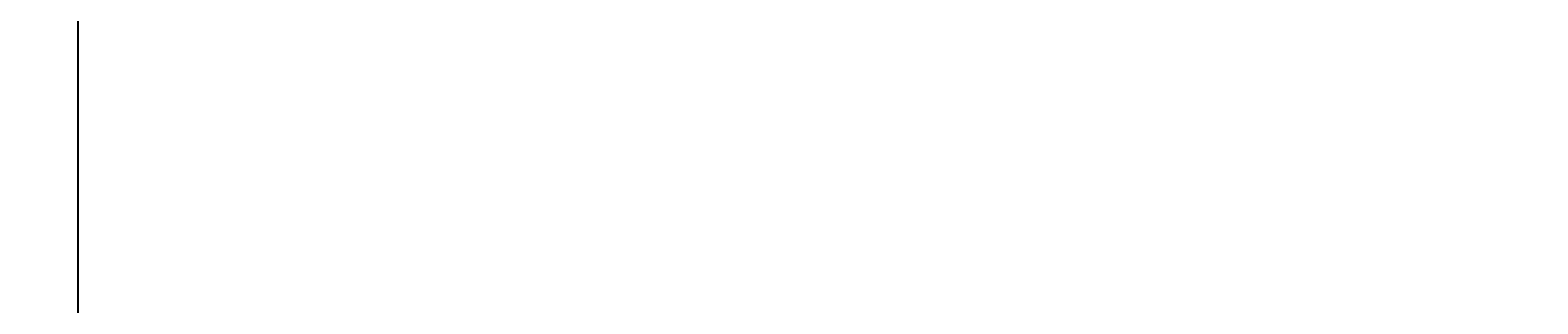
# Model space of a CAD drawing. Units: inches. Extents: x 35362 to 73946, y 43607 to 67532.
# Tile 104 of 134: x 50119 to 50761, y 49386 to 49502. Entities that reach past the tile are written whole.
import ezdxf

# ---------------------------------------------------------------- set-up
doc = ezdxf.new("R2010")
doc.units = ezdxf.units.IN
doc.header["$MEASUREMENT"] = 0
doc.layers.add('A-ANNO-DIMS', color=2, linetype='Continuous', lineweight=18)
doc.styles.get("Standard").update_dxf_attribs({"font": 'arial.ttf'})
doc.dimstyles.get("Standard").update_dxf_attribs({"dimtxt": 0.18, "dimasz": 0.18, "dimexe": 0.18, "dimexo": 0.0625, "dimgap": 0.09, "dimtad": 0, "dimtih": 1, "dimtoh": 1, "dimdec": 4, "dimzin": 0, "dimdsep": 46, "dimtxsty": 'Standard', "dimcen": 0.09, "dimadec": 0, "dimazin": 0, "dimtfac": 1, "dimtdec": 4, "dimtofl": 0, "dimtmove": 0, "dimatfit": 3, "dimfxl": 1, "dimtolj": 1, "dimtzin": 0, "dimarcsym": 0})

# ---------------------------------------------------------------- blocks, each defined once
blk = doc.blocks.new('*D11')
at = {"layer": 'A-ANNO-DIMS', "color": 0, "lineweight": -2, "transparency": 16777216}
for p, q in [((47978.66, 56028.77), (47978.66, 43606.68)), ((53109.76, 56028.77), (53109.76, 43606.68)), ((47978.84, 43606.86), (50543.87, 43606.86)), ((53109.58, 43606.86), (50544.55, 43606.86))]:
    blk.add_line(p, q, dxfattribs=at)
at = {"layer": 'A-ANNO-DIMS', "color": 0, "transparency": 16777216}
for points in [[(47978.84, 43606.89), (47978.84, 43606.83), (47978.66, 43606.86)], [(53109.58, 43606.89), (53109.58, 43606.83), (53109.76, 43606.86)]]:
    blk.add_solid(points, dxfattribs=at)
at = {"layer": 'Defpoints', "color": 0, "transparency": 16777216}
for p in [(47978.66, 56028.84), (53109.76, 56028.84), (53109.76, 43606.86)]:
    blk.add_point(p, dxfattribs=at)
at = {"layer": 'A-ANNO-DIMS', "color": 0, "transparency": 16777216, "insert": (50544.21, 43606.86), "char_height": 0.18, "attachment_point": 5}
blk.add_mtext('\\A1;5131', dxfattribs=at)
blk = doc.blocks.new('*D13')
at = {"layer": 'A-ANNO-DIMS', "color": 0, "lineweight": -2, "transparency": 16777216}
for p, q in [((48373.49, 51694.02), (48373.49, 43606.68)), ((51029.04, 51694.02), (51029.04, 43606.68)), ((48373.67, 43606.86), (49700.8, 43606.86)), ((51028.86, 43606.86), (49701.73, 43606.86))]:
    blk.add_line(p, q, dxfattribs=at)
at = {"layer": 'A-ANNO-DIMS', "color": 0, "transparency": 16777216}
for points in [[(48373.67, 43606.89), (48373.67, 43606.83), (48373.49, 43606.86)], [(51028.86, 43606.89), (51028.86, 43606.83), (51029.04, 43606.86)]]:
    blk.add_solid(points, dxfattribs=at)
at = {"layer": 'Defpoints', "color": 0, "transparency": 16777216}
for p in [(48373.49, 51694.09), (51029.04, 51694.09), (51029.04, 43606.86)]:
    blk.add_point(p, dxfattribs=at)
at = {"layer": 'A-ANNO-DIMS', "color": 0, "transparency": 16777216, "insert": (49701.27, 43606.86), "char_height": 0.18, "attachment_point": 5}
blk.add_mtext('\\A1;2655.6', dxfattribs=at)
blk = doc.blocks.new('*D17')
at = {"layer": 'A-ANNO-DIMS', "color": 0, "lineweight": -2, "transparency": 16777216}
for p, q in [((49923.31, 61293.22), (49923.31, 43606.68)), ((51913.93, 61293.22), (51913.93, 43606.68)), ((49923.49, 43606.86), (50918.16, 43606.86)), ((51913.75, 43606.86), (50919.07, 43606.86))]:
    blk.add_line(p, q, dxfattribs=at)
at = {"layer": 'A-ANNO-DIMS', "color": 0, "transparency": 16777216}
for points in [[(49923.49, 43606.89), (49923.49, 43606.83), (49923.31, 43606.86)], [(51913.75, 43606.89), (51913.75, 43606.83), (51913.93, 43606.86)]]:
    blk.add_solid(points, dxfattribs=at)
at = {"layer": 'Defpoints', "color": 0, "transparency": 16777216}
for p in [(49923.31, 61293.29), (51913.93, 61293.29), (51913.93, 43606.86)]:
    blk.add_point(p, dxfattribs=at)
at = {"layer": 'A-ANNO-DIMS', "color": 0, "transparency": 16777216, "insert": (50918.62, 43606.86), "char_height": 0.18, "attachment_point": 5}
blk.add_mtext('\\A1;1990.6', dxfattribs=at)
blk = doc.blocks.new('*D40')
at = {"layer": 'A-ANNO-DIMS', "color": 0, "lineweight": -2, "transparency": 16777216}
for p, q in [((56873.54, 53351.53), (35361.77, 53351.53)), ((35361.95, 53351.35), (35361.95, 51333.28)), ((35361.95, 49314.85), (35361.95, 51332.92)), ((51806.45, 49314.67), (35361.77, 49314.67))]:
    blk.add_line(p, q, dxfattribs=at)
at = {"layer": 'A-ANNO-DIMS', "color": 0, "transparency": 16777216}
for points in [[(35361.92, 53351.35), (35361.98, 53351.35), (35361.95, 53351.53)], [(35361.92, 49314.85), (35361.98, 49314.85), (35361.95, 49314.67)]]:
    blk.add_solid(points, dxfattribs=at)
at = {"layer": 'Defpoints', "color": 0, "transparency": 16777216}
for p in [(35361.95, 53351.53), (56873.6, 53351.53), (51806.52, 49314.67)]:
    blk.add_point(p, dxfattribs=at)
at = {"layer": 'A-ANNO-DIMS', "color": 0, "transparency": 16777216, "insert": (35361.95, 51333.1), "char_height": 0.18, "attachment_point": 5}
blk.add_mtext('\\A1;4036.9', dxfattribs=at)
blk = doc.blocks.new('*D67')
at = {"layer": 'A-ANNO-DIMS', "color": 0, "lineweight": -2, "transparency": 16777216}
for p, q in [((56873.54, 53351.53), (35361.77, 53351.53)), ((35361.95, 53351.35), (35361.95, 49400.89)), ((35361.95, 45450.07), (35361.95, 49400.53)), ((53793.58, 45449.89), (35361.77, 45449.89))]:
    blk.add_line(p, q, dxfattribs=at)
at = {"layer": 'A-ANNO-DIMS', "color": 0, "transparency": 16777216}
for points in [[(35361.92, 53351.35), (35361.98, 53351.35), (35361.95, 53351.53)], [(35361.92, 45450.07), (35361.98, 45450.07), (35361.95, 45449.89)]]:
    blk.add_solid(points, dxfattribs=at)
at = {"layer": 'Defpoints', "color": 0, "transparency": 16777216}
for p in [(35361.95, 53351.53), (56873.6, 53351.53), (53793.64, 45449.89)]:
    blk.add_point(p, dxfattribs=at)
at = {"layer": 'A-ANNO-DIMS', "color": 0, "transparency": 16777216, "insert": (35361.95, 49400.71), "char_height": 0.18, "attachment_point": 5}
blk.add_mtext('\\A1;7901.6', dxfattribs=at)
blk = doc.blocks.new('*D107')
at = {"layer": 'A-ANNO-DIMS', "color": 0, "lineweight": -2, "transparency": 16777216}
for p, q in [((50139.56, 59850.01), (50139.56, 43606.68)), ((51320.81, 59850.01), (51320.81, 43606.68)), ((50139.74, 43606.86), (50729.73, 43606.86)), ((51320.63, 43606.86), (50730.64, 43606.86))]:
    blk.add_line(p, q, dxfattribs=at)
at = {"layer": 'A-ANNO-DIMS', "color": 0, "transparency": 16777216}
for points in [[(50139.74, 43606.89), (50139.74, 43606.83), (50139.56, 43606.86)], [(51320.63, 43606.89), (51320.63, 43606.83), (51320.81, 43606.86)]]:
    blk.add_solid(points, dxfattribs=at)
at = {"layer": 'Defpoints', "color": 0, "transparency": 16777216}
for p in [(50139.56, 59850.08), (51320.81, 59850.08), (51320.81, 43606.86)]:
    blk.add_point(p, dxfattribs=at)
at = {"layer": 'A-ANNO-DIMS', "color": 0, "transparency": 16777216, "insert": (50730.19, 43606.86), "char_height": 0.18, "attachment_point": 5}
blk.add_mtext('\\A1;1181.3', dxfattribs=at)

msp = doc.modelspace()

# ---------------------------------------------------------------- dimensions: what is measured, and where the dimension line sits
at = {"layer": 'A-ANNO-DIMS'}
for base, p1, p2, override, picture, middle in [((51913.931, 43606.859), (49923.307, 61293.286), (51913.931, 61293.286), {"dimdec": 1, "dimlfac": 1, "dimrnd": 0, "dimzin": 0, "dimdsep": 46, "dimlunit": 2}, '*D17', (50918.619, 43606.859)), ((51320.8133, 43606.859), (50139.5627, 59850.0769), (51320.8133, 59850.0769), {"dimdec": 1, "dimlfac": 1, "dimrnd": 0, "dimzin": 0, "dimdsep": 46, "dimlunit": 2}, '*D107', (50730.188, 43606.859)), ((53109.76, 43606.859), (47978.665, 56028.836), (53109.76, 56028.836), {"dimdec": 0, "dimlfac": 1, "dimrnd": 0, "dimzin": 0, "dimdsep": 46, "dimlunit": 2}, '*D11', (50544.212, 43606.859)), ((51029.043, 43606.859), (48373.492, 51694.087), (51029.043, 51694.087), {"dimdec": 1, "dimlfac": 1, "dimrnd": 0, "dimzin": 0, "dimdsep": 46, "dimlunit": 2}, '*D13', (49701.267, 43606.859))]:
    dim = msp.add_linear_dim(base=base, p1=p1, p2=p2, dimstyle='Standard', override=override, dxfattribs=at)
    dim.commit()
    dim.dimension.update_dxf_attribs({"geometry": picture, "text_midpoint": middle})
for p1, picture, middle in [((51806.517, 49314.669), '*D40', (35361.949, 51333.099)), ((53793.638, 45449.894), '*D67', (35361.949, 49400.712))]:
    dim = msp.add_linear_dim(base=(35361.949, 53351.529), p1=p1, p2=(56873.602, 53351.529), angle=90, dimstyle='Standard', override={"dimdec": 1, "dimlfac": 1, "dimrnd": 0, "dimzin": 0, "dimdsep": 46, "dimlunit": 2}, dxfattribs=at)
    dim.commit()
    dim.dimension.update_dxf_attribs({"geometry": picture, "text_midpoint": middle})

doc.saveas('drawing.dxf')
